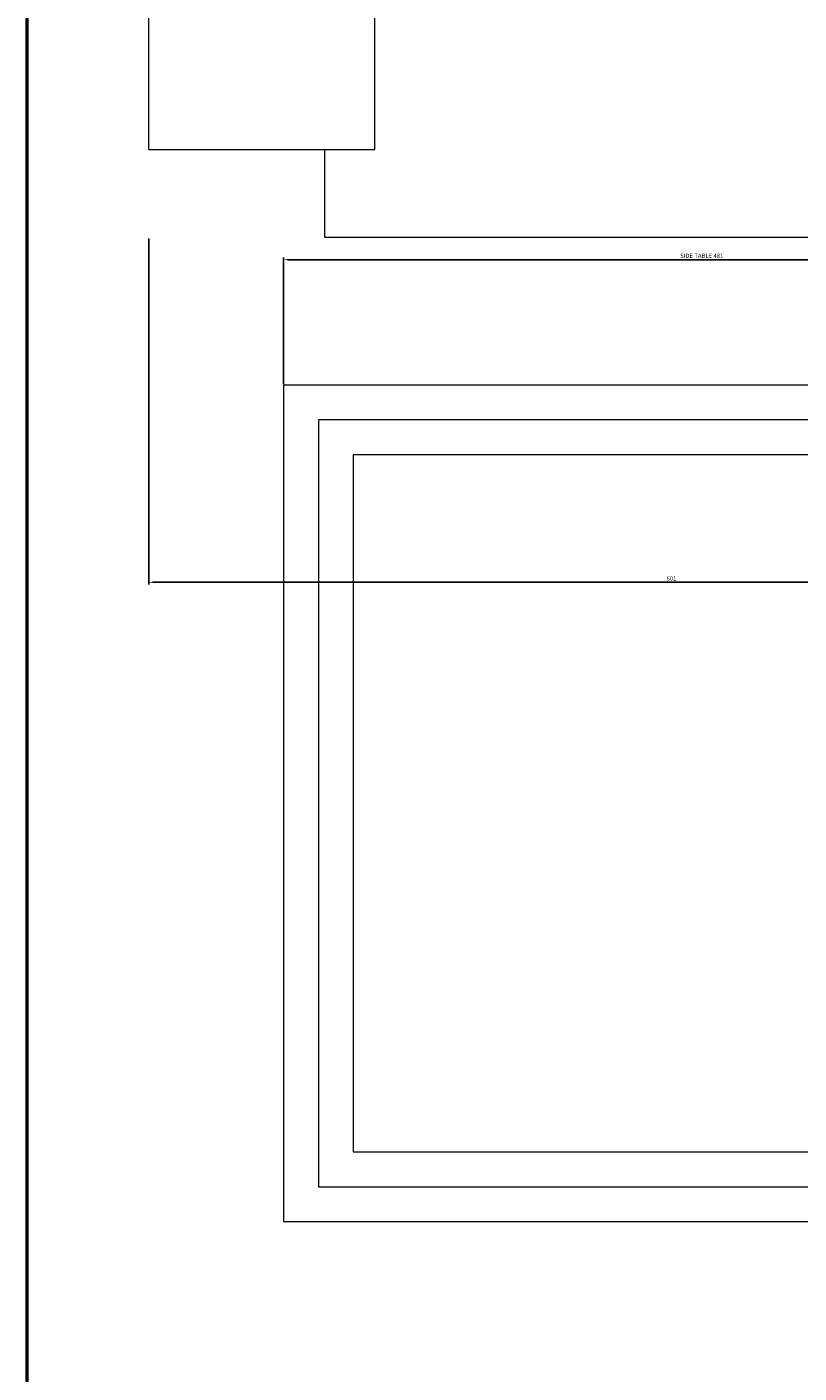
# Model space of a CAD drawing. Units: millimetres. Extents: x -857 to 54106, y -13666 to 13947.
# Tile 5 of 41: x 7417 to 7861, y 6216 to 6990. Entities that reach past the tile are written whole.
import ezdxf

# ---------------------------------------------------------------- set-up
doc = ezdxf.new("R2010")
doc.units = ezdxf.units.MM
for name, color, linetype, lineweight in [('A-ANNO-DIMS', 2, 'Continuous', 18), ('A-FURN', 21, 'Continuous', 18), ('A-FURNITURE', 25, 'Continuous', 9), ('A-WALL', 7, 'Continuous', 50)]:
    doc.layers.add(name, color=color, linetype=linetype, lineweight=lineweight)
doc.styles.get("Standard").update_dxf_attribs({"font": 'arial.ttf'})
doc.dimstyles.new('ISO-25', dxfattribs={"dimtxt": 2.5, "dimasz": 2.5, "dimexe": 1.25, "dimexo": 0.625, "dimtad": 1, "dimtxsty": 'Standard', "dimcen": 2.5, "dimadec": 0, "dimazin": 0, "dimtfac": 1, "dimtmove": 0, "dimatfit": 3, "dimfxl": 1, "dimarcsym": 0})

# ---------------------------------------------------------------- blocks, each defined once
blk = doc.blocks.new('A$C0E8E2537')
at = {"layer": 'A-FURNITURE'}
for p, q in [((30.478, 0), (-30.478, 0)), ((30.478, 0), (30.478, -6.486)), ((30.478, -5.045), (33, -5.045)), ((33, -5.045), (33, -26.997)), ((30.478, -6.486), (-30.478, -6.486))]:
    blk.add_line(p, q, dxfattribs=at)
blk = doc.blocks.new('A$C21FE29A1')
at = {"layer": 'A-FURNITURE'}
for points in [[(0, 0), (24, 0), (24, 24), (0, 24)], [(1, 1), (23, 1), (23, 23), (1, 23)], [(2, 2), (22, 2), (22, 22), (2, 22)]]:
    blk.add_lwpolyline(points, close=True, dxfattribs=at)
blk = doc.blocks.new('*D54')
at = {"layer": 'A-ANNO-DIMS', "color": 0, "lineweight": -2, "transparency": 16777216}
for p, q in [((7487.34, 6868.56), (7487.34, 6669.58)), ((8088.43, 6868.56), (8088.43, 6669.58)), ((8085.93, 6670.83), (7489.84, 6670.83))]:
    blk.add_line(p, q, dxfattribs=at)
at = {"layer": 'A-ANNO-DIMS', "color": 0, "transparency": 16777216}
for points in [[(7489.84, 6671.24), (7489.84, 6670.41), (7487.34, 6670.83)], [(8085.93, 6671.24), (8085.93, 6670.41), (8088.43, 6670.83)]]:
    blk.add_solid(points, dxfattribs=at)
at = {"layer": 'Defpoints', "color": 0, "transparency": 16777216}
for p in [(7487.34, 6869.19), (8088.43, 6869.19), (7487.34, 6670.83)]:
    blk.add_point(p, dxfattribs=at)
at = {"layer": 'A-ANNO-DIMS', "color": 0, "transparency": 16777216, "insert": (7787.89, 6672.73), "char_height": 2.5, "attachment_point": 5}
blk.add_mtext('601', dxfattribs=at)
blk = doc.blocks.new('*D57')
at = {"layer": 'A-ANNO-DIMS', "color": 0, "lineweight": -2, "transparency": 16777216}
for p, q in [((7564.88, 6784.8), (7564.88, 6857.56)), ((8045.76, 6784.8), (8045.76, 6857.56)), ((8043.26, 6856.31), (7567.38, 6856.31))]:
    blk.add_line(p, q, dxfattribs=at)
at = {"layer": 'A-ANNO-DIMS', "color": 0, "transparency": 16777216}
for points in [[(7567.38, 6856.72), (7567.38, 6855.89), (7564.88, 6856.31)], [(8043.26, 6856.72), (8043.26, 6855.89), (8045.76, 6856.31)]]:
    blk.add_solid(points, dxfattribs=at)
at = {"layer": 'Defpoints', "color": 0, "transparency": 16777216}
for p in [(7564.88, 6856.31), (7564.88, 6784.17), (8045.76, 6784.17)]:
    blk.add_point(p, dxfattribs=at)
at = {"layer": 'A-ANNO-DIMS', "color": 0, "transparency": 16777216, "insert": (7805.32, 6858.22), "char_height": 2.5, "attachment_point": 5}
blk.add_mtext('SIDE TABLE 481', dxfattribs=at)

msp = doc.modelspace()

# ---------------------------------------------------------------- linework, layer by layer
at = {"layer": 'A-WALL'}
msp.add_line((7417.28, 8154.231), (7417.28, 5554.231), dxfattribs=at)

# ---------------------------------------------------------------- block references
at = {"layer": 'A-FURN', "ltscale": 4, "xscale": -20.03650789584554, "yscale": 20.03650789584554, "zscale": 20.03650789584554, "rotation": 90}
msp.add_blockref('A$C0E8E2537', (7487.337, 7530.393), dxfattribs=at)
at = {"layer": 'A-FURN', "xscale": 20.03650789584554, "yscale": 20.03650789584554, "zscale": 20.03650789584554, "rotation": 89.99999999999999}
msp.add_blockref('A$C21FE29A1', (8045.76, 6303.297), dxfattribs=at)

# ---------------------------------------------------------------- dimensions: what is measured, and where the dimension line sits
at = {"layer": 'A-ANNO-DIMS'}
dim = msp.add_linear_dim(base=(7487.337, 6670.826), p1=(8088.433, 6869.188), p2=(7487.337, 6869.188), angle=180, dimstyle='ISO-25', override={"dimdec": 0, "dimrnd": 0, "dimzin": 0, "dimlunit": 2}, dxfattribs=at)
dim.commit()
dim.dimension.update_dxf_attribs({"geometry": '*D54', "text_midpoint": (7787.885, 6672.728)})
dim = msp.add_linear_dim(base=(7564.885, 6856.306), p1=(8045.761, 6784.175), p2=(7564.885, 6784.175), angle=180, text='SIDE TABLE <>', dimstyle='ISO-25', override={"dimdec": 0, "dimrnd": 0, "dimzin": 0, "dimlunit": 2}, dxfattribs=at)
dim.commit()
dim.dimension.update_dxf_attribs({"geometry": '*D57', "text_midpoint": (7805.323, 6858.224)})

doc.saveas('drawing.dxf')
